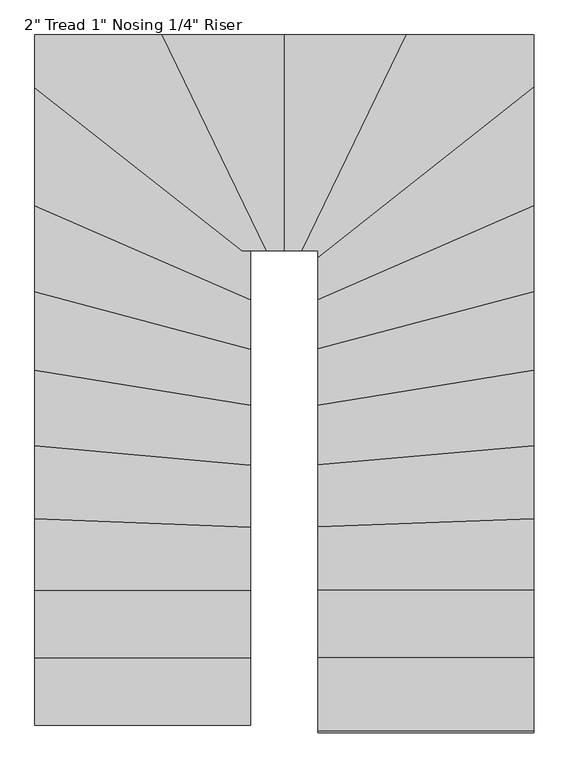
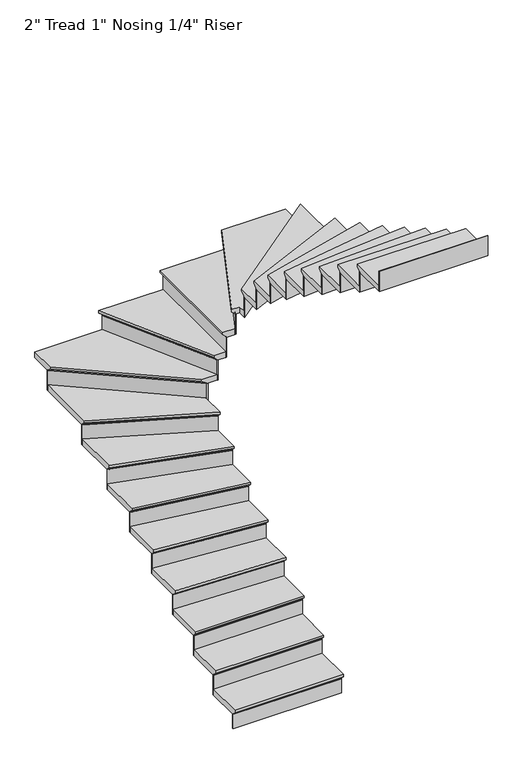
"""IFC4 building model written with IfcOpenShell, lengths in millimetres: stair flight geometry."""

from ifc_helpers import new_model, si_unit, origin, place, context, project, spatial, faceted_brep, source, transform, mapped, element, save


def stair_flight_57db1963(model_context):
    return source(origin(), model_context, "Body", "Brep", [
        faceted_brep([(-5047.1987704, -4554.2130548, 14785.5214286), (-5047.1987704, -4554.2130548, 14804.5714286), (-5940.8822214, -4554.2130548, 14804.5714286), (-5940.8822214, -4554.2130548, 14785.5214286), (-5047.1987704, -4528.8130548, 14760.1214286), (-5940.8822214, -4528.8130548, 14760.1214286), (-5047.1987704, -4249.4130548, 14804.5714286), (-5940.8822214, -4249.4130548, 14804.5714286), (-5940.8822214, -4528.8130548, 14753.7714286), (-5940.8822214, -4249.4130548, 14753.7714286), (-5047.1987704, -4249.4130548, 14753.7714286), (-5047.1987704, -4528.8130548, 14753.7714286)], [[[0, 1, 2, 3]], [[4, 0, 3, 5]], [[2, 1, 6, 7]], [[8, 9, 10, 11]], [[2, 7, 9, 8, 5, 3]], [[8, 11, 4, 5]], [[6, 1, 0, 4, 11, 10]], [[7, 6, 10, 9]]]),
        faceted_brep([(-5047.1987704, -4528.8130548, 14753.7714286), (-5047.1987704, -4528.8130548, 14630.4), (-5047.1987704, -4522.4630548, 14630.4), (-5047.1987704, -4522.4630548, 14753.7714286), (-5940.8822214, -4528.8130548, 14753.7714286), (-5940.8822214, -4522.4630548, 14753.7714286), (-5940.8822214, -4522.4630548, 14630.4), (-5940.8822214, -4528.8130548, 14630.4)], [[[0, 1, 2, 3]], [[4, 5, 6, 7]], [[1, 0, 4, 7]], [[2, 1, 7, 6]], [[3, 2, 6, 5]], [[0, 3, 5, 4]]]),
        faceted_brep([(-5047.1987704, -4249.4130548, 14927.9428571), (-5047.1987704, -4249.4130548, 14753.7714286), (-5047.1987704, -4243.0630548, 14753.7714286), (-5047.1987704, -4243.0630548, 14927.9428571), (-5940.8822214, -4249.4130548, 14927.9428571), (-5940.8822214, -4243.0630548, 14927.9428571), (-5940.8822214, -4243.0630548, 14753.7714286), (-5940.8822214, -4249.4130548, 14753.7714286)], [[[0, 1, 2, 3]], [[4, 5, 6, 7]], [[1, 0, 4, 7]], [[2, 1, 7, 6]], [[3, 2, 6, 5]], [[0, 3, 5, 4]]]),
        faceted_brep([(-5940.8822214, -4274.8130548, 14978.7428571), (-5047.1987704, -4274.8130548, 14978.7428571), (-5047.1987704, -3970.0130548, 14978.7428571), (-5940.8822214, -3970.0130548, 14978.7428571), (-5940.8822214, -4249.4130548, 14927.9428571), (-5940.8822214, -3970.0130548, 14927.9428571), (-5047.1987704, -3970.0130548, 14927.9428571), (-5047.1987704, -4249.4130548, 14927.9428571), (-5940.8822214, -4249.4130548, 14934.2928571), (-5940.8822214, -4274.8130548, 14959.6928571), (-5047.1987704, -4249.4130548, 14934.2928571), (-5047.1987704, -4274.8130548, 14959.6928571)], [[[0, 1, 2, 3]], [[4, 5, 6, 7]], [[0, 3, 5, 4, 8, 9]], [[4, 7, 10, 8]], [[2, 1, 11, 10, 7, 6]], [[3, 2, 6, 5]], [[11, 1, 0, 9]], [[10, 11, 9, 8]]]),
        faceted_brep([(-5047.1987704, -3970.0130548, 15102.1142857), (-5047.1987704, -3970.0130548, 14927.9428571), (-5047.1987704, -3963.6630548, 14927.9428571), (-5047.1987704, -3963.6630548, 15102.1142857), (-5940.8822214, -3970.0130548, 15102.1142857), (-5940.8822214, -3963.6630548, 15102.1142857), (-5940.8822214, -3963.6630548, 14927.9428571), (-5940.8822214, -3970.0130548, 14927.9428571)], [[[0, 1, 2, 3]], [[4, 5, 6, 7]], [[1, 0, 4, 7]], [[2, 1, 7, 6]], [[3, 2, 6, 5]], [[0, 3, 5, 4]]]),
        faceted_brep([(-5940.8822214, -3995.4130548, 15152.9142857), (-5047.1987704, -3995.4130548, 15152.9142857), (-5047.1987704, -3707.9036879, 15152.9142857), (-5940.8822214, -3673.2843203, 15152.9142857), (-5940.8822214, -3970.0130548, 15102.1142857), (-5940.8822214, -3673.2843203, 15102.1142857), (-5047.1987704, -3707.9036879, 15102.1142857), (-5047.1987704, -3970.0130548, 15102.1142857), (-5940.8822214, -3970.0130548, 15108.4642857), (-5940.8822214, -3995.4130548, 15133.8642857), (-5047.1987704, -3970.0130548, 15108.4642857), (-5047.1987704, -3995.4130548, 15133.8642857)], [[[0, 1, 2, 3]], [[4, 5, 6, 7]], [[0, 3, 5, 4, 8, 9]], [[4, 7, 10, 8]], [[2, 1, 11, 10, 7, 6]], [[3, 2, 6, 5]], [[11, 1, 0, 9]], [[10, 11, 9, 8]]]),
        faceted_brep([(-5047.1987704, -3707.9036879, 15276.2857143), (-5047.1987704, -3707.9036879, 15102.1142857), (-5047.1987704, -3701.5489252, 15102.1142857), (-5047.1987704, -3701.5489252, 15276.2857143), (-5940.8822214, -3673.2843203, 15276.2857143), (-5940.8822214, -3666.9295576, 15276.2857143), (-5940.8822214, -3666.9295576, 15102.1142857), (-5940.8822214, -3673.2843203, 15102.1142857)], [[[0, 1, 2, 3]], [[4, 5, 6, 7]], [[1, 0, 4, 7]], [[2, 1, 7, 6]], [[3, 2, 6, 5]], [[0, 3, 5, 4]]]),
        faceted_brep([(-5940.8822214, -3698.703371, 15327.0857143), (-5047.1987704, -3733.3227386, 15327.0857143), (-5047.1987704, -3451.3234819, 15327.0857143), (-5940.8822214, -3370.89733, 15327.0857143), (-5940.8822214, -3673.2843203, 15276.2857143), (-5940.8822214, -3370.89733, 15276.2857143), (-5047.1987704, -3451.3234819, 15276.2857143), (-5047.1987704, -3707.9036879, 15276.2857143), (-5940.8822214, -3673.2843203, 15282.6357143), (-5940.8822214, -3698.703371, 15308.0357143), (-5047.1987704, -3707.9036879, 15282.6357143), (-5047.1987704, -3733.3227386, 15308.0357143)], [[[0, 1, 2, 3]], [[4, 5, 6, 7]], [[0, 3, 5, 4, 8, 9]], [[4, 7, 10, 8]], [[2, 1, 11, 10, 7, 6]], [[3, 2, 6, 5]], [[11, 1, 0, 9]], [[10, 11, 9, 8]]]),
        faceted_brep([(-5047.1987704, -3451.3234819, 15450.4571429), (-5047.1987704, -3451.3234819, 15276.2857143), (-5047.1987704, -3444.9478197, 15276.2857143), (-5047.1987704, -3444.9478197, 15450.4571429), (-5940.8822214, -3370.89733, 15450.4571429), (-5940.8822214, -3364.5216678, 15450.4571429), (-5940.8822214, -3364.5216678, 15276.2857143), (-5940.8822214, -3370.89733, 15276.2857143)], [[[0, 1, 2, 3]], [[4, 5, 6, 7]], [[1, 0, 4, 7]], [[2, 1, 7, 6]], [[3, 2, 6, 5]], [[0, 3, 5, 4]]]),
        faceted_brep([(-5940.8822214, -3396.3999789, 15501.2571429), (-5047.1987704, -3476.8261308, 15501.2571429), (-5047.1987704, -3203.4301079, 15501.2571429), (-5940.8822214, -3059.5417727, 15501.2571429), (-5940.8822214, -3370.89733, 15450.4571429), (-5940.8822214, -3059.5417727, 15450.4571429), (-5047.1987704, -3203.4301079, 15450.4571429), (-5047.1987704, -3451.3234819, 15450.4571429), (-5940.8822214, -3370.89733, 15456.8071429), (-5940.8822214, -3396.3999789, 15482.2071429), (-5047.1987704, -3451.3234819, 15456.8071429), (-5047.1987704, -3476.8261308, 15482.2071429)], [[[0, 1, 2, 3]], [[4, 5, 6, 7]], [[0, 3, 5, 4, 8, 9]], [[4, 7, 10, 8]], [[2, 1, 11, 10, 7, 6]], [[3, 2, 6, 5]], [[11, 1, 0, 9]], [[10, 11, 9, 8]]]),
        faceted_brep([(-5047.1987704, -3203.4301079, 15624.6285714), (-5047.1987704, -3203.4301079, 15450.4571429), (-5047.1987704, -3196.9983292, 15450.4571429), (-5047.1987704, -3196.9983292, 15624.6285714), (-5940.8822214, -3059.5417727, 15624.6285714), (-5940.8822214, -3053.109994, 15624.6285714), (-5940.8822214, -3053.109994, 15450.4571429), (-5940.8822214, -3059.5417727, 15450.4571429)], [[[0, 1, 2, 3]], [[4, 5, 6, 7]], [[1, 0, 4, 7]], [[2, 1, 7, 6]], [[3, 2, 6, 5]], [[0, 3, 5, 4]]]),
        faceted_brep([(-5940.8822214, -3085.2688872, 15675.4285714), (-5047.1987704, -3229.1572224, 15675.4285714), (-5047.1987704, -2970.3553609, 15675.4285714), (-5940.8822214, -2732.7052783, 15675.4285714), (-5940.8822214, -3059.5417727, 15624.6285714), (-5940.8822214, -2732.7052783, 15624.6285714), (-5047.1987704, -2970.3553609, 15624.6285714), (-5047.1987704, -3203.4301079, 15624.6285714), (-5940.8822214, -3059.5417727, 15630.9785714), (-5940.8822214, -3085.2688872, 15656.3785714), (-5047.1987704, -3203.4301079, 15630.9785714), (-5047.1987704, -3229.1572224, 15656.3785714)], [[[0, 1, 2, 3]], [[4, 5, 6, 7]], [[0, 3, 5, 4, 8, 9]], [[4, 7, 10, 8]], [[2, 1, 11, 10, 7, 6]], [[3, 2, 6, 5]], [[11, 1, 0, 9]], [[10, 11, 9, 8]]]),
        faceted_brep([(-5047.1987704, -2970.3553609, 15798.8), (-5047.1987704, -2970.3553609, 15624.6285714), (-5047.1987704, -2963.7846771, 15624.6285714), (-5047.1987704, -2963.7846771, 15798.8), (-5940.8822214, -2732.7052783, 15798.8), (-5940.8822214, -2726.1345945, 15798.8), (-5940.8822214, -2726.1345945, 15624.6285714), (-5940.8822214, -2732.7052783, 15624.6285714)], [[[0, 1, 2, 3]], [[4, 5, 6, 7]], [[1, 0, 4, 7]], [[2, 1, 7, 6]], [[3, 2, 6, 5]], [[0, 3, 5, 4]]]),
        faceted_brep([(-5940.8822214, -2758.9880136, 15849.6), (-5047.1987704, -2996.6380961, 15849.6), (-5047.1987704, -2765.8050203, 15849.6), (-5940.8822214, -2375.5896532, 15849.6), (-5940.8822214, -2732.7052783, 15798.8), (-5940.8822214, -2375.5896532, 15798.8), (-5047.1987704, -2765.8050203, 15798.8), (-5047.1987704, -2970.3553609, 15798.8), (-5940.8822214, -2732.7052783, 15805.15), (-5940.8822214, -2758.9880136, 15830.55), (-5047.1987704, -2970.3553609, 15805.15), (-5047.1987704, -2996.6380961, 15830.55)], [[[0, 1, 2, 3]], [[4, 5, 6, 7]], [[0, 3, 5, 4, 8, 9]], [[4, 7, 10, 8]], [[2, 1, 11, 10, 7, 6]], [[3, 2, 6, 5]], [[11, 1, 0, 9]], [[10, 11, 9, 8]]]),
        faceted_brep([(-5047.1987704, -2765.8050203, 15972.9714286), (-5047.1987704, -2765.8050203, 15798.8), (-5047.1987704, -2758.8760908, 15798.8), (-5047.1987704, -2758.8760908, 15972.9714286), (-5940.8822214, -2375.5896532, 15972.9714286), (-5940.8822214, -2368.6607237, 15972.9714286), (-5940.8822214, -2368.6607237, 15798.8), (-5940.8822214, -2375.5896532, 15798.8)], [[[0, 1, 2, 3]], [[4, 5, 6, 7]], [[1, 0, 4, 7]], [[2, 1, 7, 6]], [[3, 2, 6, 5]], [[0, 3, 5, 4]]]),
        faceted_brep([(-5940.8822214, -2403.3053713, 16023.7714286), (-5047.1987704, -2793.5207384, 16023.7714286), (-5047.1987704, -2590.8424524, 16023.7714286), (-5040.8038639, -2590.8424524, 16023.7714286), (-5940.8822214, -1882.1944717, 16023.7714286), (-5940.8822214, -2375.5896532, 15972.9714286), (-5940.8822214, -1882.1944717, 15972.9714286), (-5040.8038639, -2590.8424524, 15972.9714286), (-5047.1987704, -2590.8424524, 15972.9714286), (-5047.1987704, -2765.8050203, 15972.9714286), (-5940.8822214, -2375.5896532, 15979.3214286), (-5940.8822214, -2403.3053713, 16004.7214286), (-5047.1987704, -2765.8050203, 15979.3214286), (-5047.1987704, -2793.5207384, 16004.7214286)], [[[0, 1, 2, 3, 4]], [[5, 6, 7, 8, 9]], [[0, 4, 6, 5, 10, 11]], [[5, 9, 12, 10]], [[2, 1, 13, 12, 9, 8]], [[4, 3, 7, 6]], [[13, 1, 0, 11]], [[12, 13, 11, 10]], [[3, 2, 8, 7]]]),
        faceted_brep([(-5040.8038639, -2590.8424524, 16147.1428571), (-5040.8038639, -2590.8424524, 15972.9714286), (-5030.5387554, -2590.8424524, 15972.9714286), (-5030.5387554, -2590.8424524, 16147.1428571), (-5940.8822214, -1882.1944717, 16147.1428571), (-5940.8822214, -1874.1125661, 16147.1428571), (-5940.8822214, -1874.1125661, 15972.9714286), (-5940.8822214, -1882.1944717, 15972.9714286)], [[[0, 1, 2, 3]], [[4, 5, 6, 7]], [[1, 0, 4, 7]], [[2, 1, 7, 6]], [[3, 2, 6, 5]], [[0, 3, 5, 4]]]),
        faceted_brep([(-5384.6489457, -1697.1590014, 16197.9428571), (-5940.8822214, -1697.1590014, 16197.9428571), (-5940.8822214, -1914.5220945, 16197.9428571), (-5081.8642978, -2590.8424524, 16197.9428571), (-4952.3566185, -2590.8424524, 16197.9428571), (-5940.8822214, -1697.1590014, 16147.1428571), (-5384.6489457, -1697.1590014, 16147.1428571), (-4952.3566185, -2590.8424524, 16147.1428571), (-5040.8038639, -2590.8424524, 16147.1428571), (-5940.8822214, -1882.1944717, 16147.1428571), (-5940.8822214, -1882.1944717, 16153.4928571), (-5940.8822214, -1914.5220945, 16178.8928571), (-5040.8038639, -2590.8424524, 16153.4928571), (-5081.8642978, -2590.8424524, 16178.8928571)], [[[0, 1, 2, 3, 4]], [[5, 6, 7, 8, 9]], [[1, 0, 6, 5]], [[2, 1, 5, 9, 10, 11]], [[9, 8, 12, 10]], [[4, 3, 13, 12, 8, 7]], [[0, 4, 7, 6]], [[13, 3, 2, 11]], [[12, 13, 11, 10]]]),
        faceted_brep([(-4952.3566185, -2590.8424524, 16321.3142857), (-4952.3566185, -2590.8424524, 16147.1428571), (-4945.3027294, -2590.8424524, 16147.1428571), (-4945.3027294, -2590.8424524, 16321.3142857), (-5384.6489457, -1697.1590014, 16321.3142857), (-5377.5950566, -1697.1590014, 16321.3142857), (-5377.5950566, -1697.1590014, 16147.1428571), (-5384.6489457, -1697.1590014, 16147.1428571)], [[[0, 1, 2, 3]], [[4, 5, 6, 7]], [[1, 0, 4, 7]], [[2, 1, 7, 6]], [[3, 2, 6, 5]], [[0, 3, 5, 4]]]),
        faceted_brep([(-5412.8645022, -1697.1590014, 16372.1142857), (-4980.5721749, -2590.8424524, 16372.1142857), (-4882.0987704, -2590.8424524, 16372.1142857), (-4882.0987706, -1697.1590014, 16372.1142857), (-5384.6489457, -1697.1590014, 16321.3142857), (-4882.0987706, -1697.1590014, 16321.3142857), (-4882.0987704, -2590.8424524, 16321.3142857), (-4952.3566185, -2590.8424524, 16321.3142857), (-5384.6489457, -1697.1590014, 16327.6642857), (-5412.8645022, -1697.1590014, 16353.0642857), (-4952.3566185, -2590.8424524, 16327.6642857), (-4980.5721749, -2590.8424524, 16353.0642857)], [[[0, 1, 2, 3]], [[4, 5, 6, 7]], [[0, 3, 5, 4, 8, 9]], [[4, 7, 10, 8]], [[3, 2, 6, 5]], [[11, 1, 0, 9]], [[10, 11, 9, 8]], [[2, 1, 11, 10, 7, 6]]]),
        faceted_brep([(-4882.0987704, -2590.8424524, 16495.4857143), (-4882.0987704, -2590.8424524, 16321.3142857), (-4875.7487704, -2590.8424524, 16321.3142857), (-4875.7487704, -2590.8424524, 16495.4857143), (-4882.0987706, -1697.1590014, 16495.4857143), (-4875.7487706, -1697.1590014, 16495.4857143), (-4875.7487706, -1697.1590014, 16321.3142857), (-4882.0987706, -1697.1590014, 16321.3142857)], [[[0, 1, 2, 3]], [[4, 5, 6, 7]], [[1, 0, 4, 7]], [[2, 1, 7, 6]], [[3, 2, 6, 5]], [[0, 3, 5, 4]]]),
        faceted_brep([(-4907.4987706, -1697.1590014, 16546.2857143), (-4907.4987704, -2590.8424524, 16546.2857143), (-4806.2098095, -2590.8424524, 16546.2857143), (-4373.9174828, -1697.1590014, 16546.2857143), (-4882.0987706, -1697.1590014, 16495.4857143), (-4373.9174828, -1697.1590014, 16495.4857143), (-4806.2098095, -2590.8424524, 16495.4857143), (-4882.0987704, -2590.8424524, 16495.4857143), (-4882.0987706, -1697.1590014, 16501.8357143), (-4907.4987706, -1697.1590014, 16527.2357143), (-4882.0987704, -2590.8424524, 16501.8357143), (-4907.4987704, -2590.8424524, 16527.2357143)], [[[0, 1, 2, 3]], [[4, 5, 6, 7]], [[0, 3, 5, 4, 8, 9]], [[4, 7, 10, 8]], [[2, 1, 11, 10, 7, 6]], [[3, 2, 6, 5]], [[11, 1, 0, 9]], [[10, 11, 9, 8]]]),
        faceted_brep([(-4806.2098095, -2590.8424524, 16669.6571429), (-4806.2098095, -2590.8424524, 16495.4857143), (-4799.1559204, -2590.8424524, 16495.4857143), (-4799.1559204, -2590.8424524, 16669.6571429), (-4373.9174828, -1697.1590014, 16669.6571429), (-4366.8635937, -1697.1590014, 16669.6571429), (-4366.8635937, -1697.1590014, 16495.4857143), (-4373.9174828, -1697.1590014, 16495.4857143)], [[[0, 1, 2, 3]], [[4, 5, 6, 7]], [[1, 0, 4, 7]], [[2, 1, 7, 6]], [[3, 2, 6, 5]], [[0, 3, 5, 4]]]),
        faceted_brep([(-3874.1153195, -1946.8497166, 16720.4571429), (-3874.1153195, -1697.1590014, 16720.4571429), (-4402.1330392, -1697.1590014, 16720.4571429), (-4834.4253659, -2590.8424524, 16720.4571429), (-4767.7987704, -2590.8424524, 16720.4571429), (-4767.7987704, -2650.4628721, 16720.4571429), (-3874.1153195, -1697.1590014, 16669.6571429), (-3874.1153195, -1946.8497166, 16669.6571429), (-4767.7987704, -2650.4628721, 16669.6571429), (-4767.7987704, -2590.8424524, 16669.6571429), (-4806.2098095, -2590.8424524, 16669.6571429), (-4373.9174828, -1697.1590014, 16669.6571429), (-4806.2098095, -2590.8424524, 16676.0071429), (-4373.9174828, -1697.1590014, 16676.0071429), (-4834.4253659, -2590.8424524, 16701.4071429), (-4402.1330392, -1697.1590014, 16701.4071429)], [[[0, 1, 2, 3, 4, 5]], [[6, 7, 8, 9, 10, 11]], [[1, 0, 7, 6]], [[11, 10, 12, 13]], [[4, 3, 14, 12, 10, 9]], [[5, 4, 9, 8]], [[0, 5, 8, 7]], [[14, 3, 2, 15]], [[12, 14, 15, 13]], [[2, 1, 6, 11, 13, 15]]]),
        faceted_brep([(-4767.7987704, -2650.4628721, 16843.8285714), (-4767.7987704, -2650.4628721, 16669.6571429), (-4767.7987704, -2658.5447778, 16669.6571429), (-4767.7987704, -2658.5447778, 16843.8285714), (-3874.1153195, -1946.8497166, 16843.8285714), (-3874.1153195, -1954.9316222, 16843.8285714), (-3874.1153195, -1954.9316222, 16669.6571429), (-3874.1153195, -1946.8497166, 16669.6571429)], [[[0, 1, 2, 3]], [[4, 5, 6, 7]], [[1, 0, 4, 7]], [[2, 1, 7, 6]], [[3, 2, 6, 5]], [[0, 3, 5, 4]]]),
        faceted_brep([(-3874.1153195, -1914.5220938, 16894.6285714), (-4767.7987704, -2618.1352494, 16894.6285714), (-4767.7987704, -2821.2364563, 16894.6285714), (-3874.1153195, -2431.0210889, 16894.6285714), (-3874.1153195, -1946.8497166, 16843.8285714), (-3874.1153195, -2431.0210889, 16843.8285714), (-4767.7987704, -2821.2364563, 16843.8285714), (-4767.7987704, -2650.4628721, 16843.8285714), (-3874.1153195, -1946.8497166, 16850.1785714), (-3874.1153195, -1914.5220938, 16875.5785714), (-4767.7987704, -2650.4628721, 16850.1785714), (-4767.7987704, -2618.1352494, 16875.5785714)], [[[0, 1, 2, 3]], [[4, 5, 6, 7]], [[0, 3, 5, 4, 8, 9]], [[4, 7, 10, 8]], [[2, 1, 11, 10, 7, 6]], [[3, 2, 6, 5]], [[11, 1, 0, 9]], [[10, 11, 9, 8]]]),
        faceted_brep([(-4767.7987704, -2821.2364563, 17018.0), (-4767.7987704, -2821.2364563, 16843.8285714), (-4767.7987704, -2828.1653858, 16843.8285714), (-4767.7987704, -2828.1653858, 17018.0), (-3874.1153195, -2431.0210889, 17018.0), (-3874.1153195, -2437.9500185, 17018.0), (-3874.1153195, -2437.9500185, 16843.8285714), (-3874.1153195, -2431.0210889, 16843.8285714)], [[[0, 1, 2, 3]], [[4, 5, 6, 7]], [[1, 0, 4, 7]], [[2, 1, 7, 6]], [[3, 2, 6, 5]], [[0, 3, 5, 4]]]),
        faceted_brep([(-3874.1153195, -2403.3053709, 17068.8), (-4767.7987704, -2793.5207382, 17068.8), (-4767.7987704, -3022.9208311, 17068.8), (-3874.1153195, -2785.2707484, 17068.8), (-3874.1153195, -2431.0210889, 17018.0), (-3874.1153195, -2785.2707484, 17018.0), (-4767.7987704, -3022.9208311, 17018.0), (-4767.7987704, -2821.2364563, 17018.0), (-3874.1153195, -2431.0210889, 17024.35), (-3874.1153195, -2403.3053709, 17049.75), (-4767.7987704, -2821.2364563, 17024.35), (-4767.7987704, -2793.5207382, 17049.75)], [[[0, 1, 2, 3]], [[4, 5, 6, 7]], [[0, 3, 5, 4, 8, 9]], [[4, 7, 10, 8]], [[2, 1, 11, 10, 7, 6]], [[3, 2, 6, 5]], [[11, 1, 0, 9]], [[10, 11, 9, 8]]]),
        faceted_brep([(-4767.7987704, -3022.9208311, 17192.1714286), (-4767.7987704, -3022.9208311, 17018.0), (-4767.7987704, -3029.4915149, 17018.0), (-4767.7987704, -3029.4915149, 17192.1714286), (-3874.1153195, -2785.2707484, 17192.1714286), (-3874.1153195, -2791.8414322, 17192.1714286), (-3874.1153195, -2791.8414322, 17018.0), (-3874.1153195, -2785.2707484, 17018.0)], [[[0, 1, 2, 3]], [[4, 5, 6, 7]], [[1, 0, 4, 7]], [[2, 1, 7, 6]], [[3, 2, 6, 5]], [[0, 3, 5, 4]]]),
        faceted_brep([(-3874.1153195, -2758.9880132, 17242.9714286), (-4767.7987704, -2996.6380959, 17242.9714286), (-4767.7987704, -3254.8843368, 17242.9714286), (-3874.1153195, -3110.9960015, 17242.9714286), (-3874.1153195, -2785.2707484, 17192.1714286), (-3874.1153195, -3110.9960015, 17192.1714286), (-4767.7987704, -3254.8843368, 17192.1714286), (-4767.7987704, -3022.9208311, 17192.1714286), (-3874.1153195, -2785.2707484, 17198.5214286), (-3874.1153195, -2758.9880132, 17223.9214286), (-4767.7987704, -3022.9208311, 17198.5214286), (-4767.7987704, -2996.6380959, 17223.9214286)], [[[0, 1, 2, 3]], [[4, 5, 6, 7]], [[0, 3, 5, 4, 8, 9]], [[4, 7, 10, 8]], [[2, 1, 11, 10, 7, 6]], [[3, 2, 6, 5]], [[11, 1, 0, 9]], [[10, 11, 9, 8]]]),
        faceted_brep([(-4767.7987704, -3254.8843368, 17366.3428571), (-4767.7987704, -3254.8843368, 17192.1714286), (-4767.7987704, -3261.3161154, 17192.1714286), (-4767.7987704, -3261.3161154, 17366.3428571), (-3874.1153195, -3110.9960015, 17366.3428571), (-3874.1153195, -3117.4277801, 17366.3428571), (-3874.1153195, -3117.4277801, 17192.1714286), (-3874.1153195, -3110.9960015, 17192.1714286)], [[[0, 1, 2, 3]], [[4, 5, 6, 7]], [[1, 0, 4, 7]], [[2, 1, 7, 6]], [[3, 2, 6, 5]], [[0, 3, 5, 4]]]),
        faceted_brep([(-3874.1153195, -3085.2688869, 17417.1428571), (-4767.7987704, -3229.1572222, 17417.1428571), (-4767.7987704, -3502.3287795, 17417.1428571), (-3874.1153195, -3421.9026274, 17417.1428571), (-3874.1153195, -3110.9960015, 17366.3428571), (-3874.1153195, -3421.9026274, 17366.3428571), (-4767.7987704, -3502.3287795, 17366.3428571), (-4767.7987704, -3254.8843368, 17366.3428571), (-3874.1153195, -3110.9960015, 17372.6928571), (-3874.1153195, -3085.2688869, 17398.0928571), (-4767.7987704, -3254.8843368, 17372.6928571), (-4767.7987704, -3229.1572222, 17398.0928571)], [[[0, 1, 2, 3]], [[4, 5, 6, 7]], [[0, 3, 5, 4, 8, 9]], [[4, 7, 10, 8]], [[2, 1, 11, 10, 7, 6]], [[3, 2, 6, 5]], [[11, 1, 0, 9]], [[10, 11, 9, 8]]]),
        faceted_brep([(-4767.7987704, -3502.3287795, 17540.5142857), (-4767.7987704, -3502.3287795, 17366.3428571), (-4767.7987704, -3508.7044417, 17366.3428571), (-4767.7987704, -3508.7044417, 17540.5142857), (-3874.1153195, -3421.9026274, 17540.5142857), (-3874.1153195, -3428.2782897, 17540.5142857), (-3874.1153195, -3428.2782897, 17366.3428571), (-3874.1153195, -3421.9026274, 17366.3428571)], [[[0, 1, 2, 3]], [[4, 5, 6, 7]], [[1, 0, 4, 7]], [[2, 1, 7, 6]], [[3, 2, 6, 5]], [[0, 3, 5, 4]]]),
        faceted_brep([(-3874.1153195, -3396.3999786, 17591.3142857), (-4767.7987704, -3476.8261306, 17591.3142857), (-4767.7987704, -3758.7417891, 17591.3142857), (-3874.1153195, -3724.1224215, 17591.3142857), (-3874.1153195, -3421.9026274, 17540.5142857), (-3874.1153195, -3724.1224215, 17540.5142857), (-4767.7987704, -3758.7417891, 17540.5142857), (-4767.7987704, -3502.3287795, 17540.5142857), (-3874.1153195, -3421.9026274, 17546.8642857), (-3874.1153195, -3396.3999786, 17572.2642857), (-4767.7987704, -3502.3287795, 17546.8642857), (-4767.7987704, -3476.8261306, 17572.2642857)], [[[0, 1, 2, 3]], [[4, 5, 6, 7]], [[0, 3, 5, 4, 8, 9]], [[4, 7, 10, 8]], [[2, 1, 11, 10, 7, 6]], [[3, 2, 6, 5]], [[11, 1, 0, 9]], [[10, 11, 9, 8]]]),
        faceted_brep([(-4767.7987704, -3758.7417891, 17714.6857143), (-4767.7987704, -3758.7417891, 17540.5142857), (-4767.7987704, -3765.0965518, 17540.5142857), (-4767.7987704, -3765.0965518, 17714.6857143), (-3874.1153195, -3724.1224215, 17714.6857143), (-3874.1153195, -3730.4771842, 17714.6857143), (-3874.1153195, -3730.4771842, 17540.5142857), (-3874.1153195, -3724.1224215, 17540.5142857)], [[[0, 1, 2, 3]], [[4, 5, 6, 7]], [[1, 0, 4, 7]], [[2, 1, 7, 6]], [[3, 2, 6, 5]], [[0, 3, 5, 4]]]),
        faceted_brep([(-3874.1153195, -3698.7033708, 17765.4857143), (-4767.7987704, -3733.3227384, 17765.4857143), (-4767.7987704, -4020.8130546, 17765.4857143), (-3874.1153195, -4020.8130546, 17765.4857143), (-3874.1153195, -3724.1224215, 17714.6857143), (-3874.1153195, -4020.8130546, 17714.6857143), (-4767.7987704, -4020.8130546, 17714.6857143), (-4767.7987704, -3758.7417891, 17714.6857143), (-3874.1153195, -3724.1224215, 17721.0357143), (-3874.1153195, -3698.7033708, 17746.4357143), (-4767.7987704, -3758.7417891, 17721.0357143), (-4767.7987704, -3733.3227384, 17746.4357143)], [[[0, 1, 2, 3]], [[4, 5, 6, 7]], [[0, 3, 5, 4, 8, 9]], [[4, 7, 10, 8]], [[2, 1, 11, 10, 7, 6]], [[3, 2, 6, 5]], [[11, 1, 0, 9]], [[10, 11, 9, 8]]]),
        faceted_brep([(-4767.7987704, -4020.8130546, 17888.8571429), (-4767.7987704, -4020.8130546, 17714.6857143), (-4767.7987704, -4027.1630546, 17714.6857143), (-4767.7987704, -4027.1630546, 17888.8571429), (-3874.1153195, -4020.8130546, 17888.8571429), (-3874.1153195, -4027.1630546, 17888.8571429), (-3874.1153195, -4027.1630546, 17714.6857143), (-3874.1153195, -4020.8130546, 17714.6857143)], [[[0, 1, 2, 3]], [[4, 5, 6, 7]], [[1, 0, 4, 7]], [[2, 1, 7, 6]], [[3, 2, 6, 5]], [[0, 3, 5, 4]]]),
        faceted_brep([(-3874.1153195, -3995.4130546, 17939.6571429), (-4767.7987704, -3995.4130546, 17939.6571429), (-4767.7987704, -4300.2130546, 17939.6571429), (-3874.1153195, -4300.2130546, 17939.6571429), (-3874.1153195, -4020.8130546, 17888.8571429), (-3874.1153195, -4300.2130546, 17888.8571429), (-4767.7987704, -4300.2130546, 17888.8571429), (-4767.7987704, -4020.8130546, 17888.8571429), (-3874.1153195, -4020.8130546, 17895.2071429), (-3874.1153195, -3995.4130546, 17920.6071429), (-4767.7987704, -4020.8130546, 17895.2071429), (-4767.7987704, -3995.4130546, 17920.6071429)], [[[0, 1, 2, 3]], [[4, 5, 6, 7]], [[0, 3, 5, 4, 8, 9]], [[4, 7, 10, 8]], [[2, 1, 11, 10, 7, 6]], [[3, 2, 6, 5]], [[11, 1, 0, 9]], [[10, 11, 9, 8]]]),
        faceted_brep([(-4767.7987704, -4300.2130546, 18063.0285714), (-4767.7987704, -4300.2130546, 17888.8571429), (-4767.7987704, -4306.5630546, 17888.8571429), (-4767.7987704, -4306.5630546, 18063.0285714), (-3874.1153195, -4300.2130546, 18063.0285714), (-3874.1153195, -4306.5630546, 18063.0285714), (-3874.1153195, -4306.5630546, 17888.8571429), (-3874.1153195, -4300.2130546, 17888.8571429)], [[[0, 1, 2, 3]], [[4, 5, 6, 7]], [[1, 0, 4, 7]], [[2, 1, 7, 6]], [[3, 2, 6, 5]], [[0, 3, 5, 4]]]),
        faceted_brep([(-4767.7987704, -4579.6130546, 18237.2), (-4767.7987704, -4579.6130546, 18063.0285714), (-4767.7987704, -4585.9630546, 18063.0285714), (-4767.7987704, -4585.9630546, 18237.2), (-3874.1153195, -4579.6130546, 18237.2), (-3874.1153195, -4585.9630546, 18237.2), (-3874.1153195, -4585.9630546, 18063.0285714), (-3874.1153195, -4579.6130546, 18063.0285714)], [[[0, 1, 2, 3]], [[4, 5, 6, 7]], [[1, 0, 4, 7]], [[2, 1, 7, 6]], [[3, 2, 6, 5]], [[0, 3, 5, 4]]]),
        faceted_brep([(-3874.1153195, -4274.8130546, 18113.8285714), (-4767.7987704, -4274.8130546, 18113.8285714), (-4767.7987704, -4579.6130546, 18113.8285714), (-3874.1153195, -4579.6130546, 18113.8285714), (-3874.1153195, -4300.2130546, 18063.0285714), (-3874.1153195, -4579.6130546, 18063.0285714), (-4767.7987704, -4579.6130546, 18063.0285714), (-4767.7987704, -4300.2130546, 18063.0285714), (-3874.1153195, -4300.2130546, 18069.3785714), (-3874.1153195, -4274.8130546, 18094.7785714), (-4767.7987704, -4300.2130546, 18069.3785714), (-4767.7987704, -4274.8130546, 18094.7785714)], [[[0, 1, 2, 3]], [[4, 5, 6, 7]], [[0, 3, 5, 4, 8, 9]], [[4, 7, 10, 8]], [[2, 1, 11, 10, 7, 6]], [[3, 2, 6, 5]], [[11, 1, 0, 9]], [[10, 11, 9, 8]]]),
    ])


if __name__ == "__main__":
    model = new_model("IFC4")
    model_context = context("Model", 3, world=origin())
    ifc_project = project(units=[si_unit("LENGTHUNIT", "METRE", prefix="MILLI")], contexts=[model_context])
    site = spatial("IfcSite", under=ifc_project)
    building = spatial("IfcBuilding", under=site)
    placement = place(None, origin())
    stair_flight_shape = stair_flight_57db1963(model_context)
    element("IfcStairFlight", 1, ObjectType="2\" Tread 1\" Nosing 1/4\" Riser", at=placement, inside=building, context=model_context, shape_type="MappedRepresentation", body=[
        mapped(stair_flight_shape, transform((0.0, 0.0, 0.0), x_axis=(1.0, 0.0, 0.0), y_axis=(0.0, 1.0, 0.0), z_axis=(0.0, 0.0, 1.0))),
    ])
    save(model, "model.ifc")

# Revit data of these elements
# Element 1 (IfcStairFlight, "2\" Tread 1\" Nosing 1/4\" Riser")
#   Materials on its faces: "Tile, Porcelain, 4in"
# Materials
#   "Tile, Porcelain, 4in": class "Generic", colour RGB 89 87 158, transparency 0, Description = "Porcelain tile, 4\", white", Cost = 0
